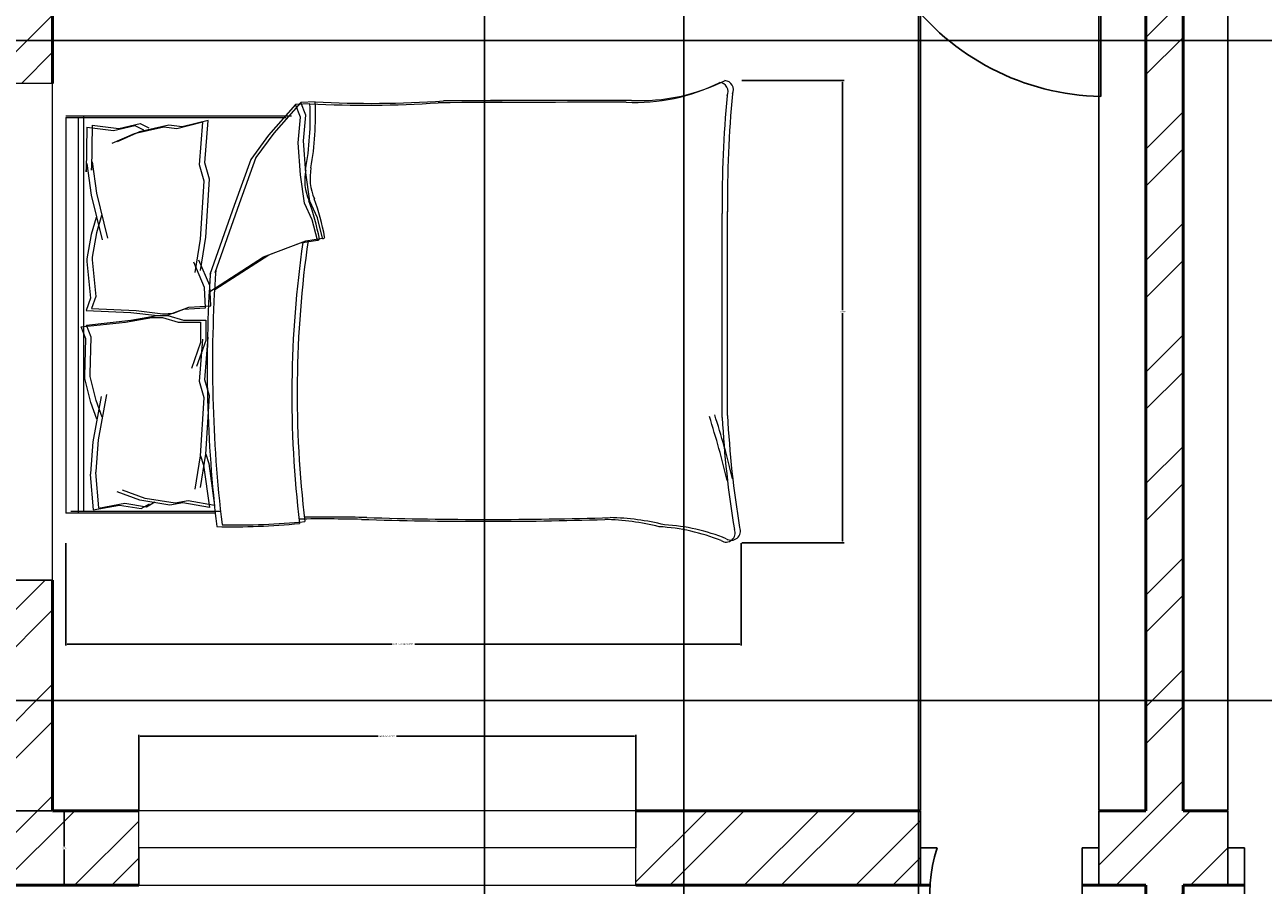
# Model space of a CAD drawing. Units: inches. Extents: x 1980 to 2738, y 1471 to 2568.
# Tile 3 of 22: x 2111 to 2260, y 1686 to 1790. Entities that reach past the tile are written whole.
import ezdxf

# ---------------------------------------------------------------- set-up
doc = ezdxf.new("R2010")
doc.units = ezdxf.units.IN
for name, color, linetype, lineweight in [('A-ANNO-DIMS', 2, 'Continuous', 18), ('A-DOOR', 31, 'Continuous', 25), ('A-FURN', 8, 'Continuous', 18), ('A-GLAZ', 141, 'Continuous', 18), ('A-WALL', 7, 'Continuous', 50)]:
    doc.layers.add(name, color=color, linetype=linetype, lineweight=lineweight)
doc.layers.add('A-WALL-PATT', color=9, linetype='Continuous', lineweight=13, true_color=0xd19cc7)
doc.styles.get("Standard").update_dxf_attribs({"font": 'arial.ttf'})
doc.dimstyles.get("Standard").update_dxf_attribs({"dimtxt": 0.18, "dimasz": 0.18, "dimexe": 0.18, "dimexo": 0.0625, "dimgap": 0.09, "dimtad": 0, "dimtih": 1, "dimtoh": 1, "dimdec": 4, "dimzin": 0, "dimdsep": 46, "dimtxsty": 'Standard', "dimcen": 0.09, "dimadec": 0, "dimazin": 0, "dimtfac": 1, "dimtdec": 4, "dimtofl": 0, "dimtmove": 0, "dimatfit": 3, "dimfxl": 1, "dimtolj": 1, "dimtzin": 0, "dimarcsym": 0})

# ---------------------------------------------------------------- blocks, each defined once
blk = doc.blocks.new('BED-DOUBLE')
for p, q in [((27.75, 52.87), (24.5, 49.16)), ((27.75, 52.87), (24.5, 49.16)), ((28.38, 53.1), (25.13, 49.39)), ((28.38, 53.1), (25.13, 49.39)), ((29.49, 52.95), (27.75, 52.87, 3.87)), ((29.49, 52.95), (27.75, 52.87, 3.87)), ((28.36, 51.33), (27.75, 52.87)), ((28.36, 51.33), (27.75, 52.87)), ((30.13, 53.18), (28.38, 53.1, 3.87)), ((30.13, 53.18), (28.38, 53.1, 3.87)), ((29, 51.56), (28.38, 53.1)), ((29, 51.56), (28.38, 53.1)), ((0, 51.49), (0.64, 51.49)), ((0, 51.27), (26.61, 51.27)), ((0, 51.27), (26.61, 51.27)), ((0, 51.27), (0, 3.48)), ((0.64, 51.49), (27.25, 51.49)), ((0.64, 51.49), (27.25, 51.49)), ((1.53, 3.48), (1.53, 51.27)), ((1.53, 3.48), (1.53, 51.27)), ((2.17, 3.7), (2.17, 51.49)), ((2.17, 3.7), (2.17, 51.49)), ((17.21, 50.93), (14.07, 50.15)), ((17.21, 50.93), (14.07, 50.15)), ((16.81, 45.8), (17.21, 50.93)), ((16.81, 45.79), (17.21, 50.93)), ((28.06, 48.23), (28.36, 51.33)), ((28.06, 48.23), (28.36, 51.33)), ((28.69, 48.46), (29, 51.56)), ((28.69, 48.46), (29, 51.56)), ((2.56, 50.11), (2.46, 44.71)), ((2.56, 50.11), (2.46, 44.71)), ((2.56, 50.11), (5.77, 49.73)), ((2.56, 50.11), (5.77, 49.73)), ((3.2, 50.34), (3.1, 44.94)), ((3.2, 50.34), (3.1, 44.94)), ((3.2, 50.34), (6.41, 49.96)), ((3.2, 50.34), (6.41, 49.96)), ((5.77, 49.73), (8.34, 50.33)), ((5.77, 49.73), (8.34, 50.33)), ((8.9, 49.54), (6.22, 48.36)), ((8.9, 49.54), (6.22, 48.36)), ((6.41, 49.96), (8.98, 50.56)), ((6.41, 49.96), (8.98, 50.56)), ((11.83, 50.11), (8.26, 49.31)), ((11.83, 50.11), (8.26, 49.31)), ((8.34, 50.33), (9.38, 49.81)), ((8.34, 50.33), (9.38, 49.81)), ((12.47, 50.34), (8.9, 49.54)), ((12.47, 50.34), (8.9, 49.54)), ((8.98, 50.56), (10.02, 50.04)), ((8.98, 50.56), (10.02, 50.04)), ((13.43, 49.92), (11.83, 50.11)), ((13.43, 49.92), (11.83, 50.11)), ((14.07, 50.15), (12.47, 50.34)), ((14.07, 50.15), (12.47, 50.34)), ((16.57, 50.7), (13.43, 49.92)), ((16.57, 50.7), (13.43, 49.92)), ((16.17, 45.57), (16.57, 50.7)), ((16.17, 45.57), (16.57, 50.7)), ((25.13, 49.39), (22.97, 46.45)), ((25.13, 49.39), (22.97, 46.45)), ((8.26, 49.31), (5.58, 48.13)), ((8.26, 49.31), (5.58, 48.13)), ((24.5, 49.16), (22.33, 46.22)), ((24.5, 49.16), (22.33, 46.22)), ((28.36, 44.36), (28.06, 48.23)), ((28.36, 44.36), (28.06, 48.23)), ((29, 44.59), (28.69, 48.46)), ((29, 44.59), (28.69, 48.46)), ((22.97, 46.45), (20.96, 40.87)), ((22.97, 46.45), (20.96, 40.87)), ((2.46, 44.71), (2.54, 45.71)), ((2.46, 44.71), (2.54, 45.71)), ((2.54, 45.71), (3.07, 41.91)), ((2.54, 45.71), (3.07, 41.91)), ((3.1, 44.94), (3.18, 45.94)), ((3.1, 44.94), (3.18, 45.94)), ((3.18, 45.94), (3.71, 42.14)), ((3.18, 45.94), (3.71, 42.14)), ((16.73, 43.61), (16.17, 45.57)), ((16.73, 43.61), (16.17, 45.57)), ((17.37, 43.83), (16.81, 45.8)), ((17.37, 43.83), (16.81, 45.79)), ((22.33, 46.22), (20.32, 40.64)), ((22.33, 46.22), (20.32, 40.64)), ((16.29, 36.6), (16.73, 43.61)), ((16.29, 36.6), (16.73, 43.61)), ((16.93, 36.82), (17.37, 43.83)), ((16.93, 36.82), (17.37, 43.83)), ((28.83, 40.95), (28.36, 44.36)), ((28.83, 40.95), (28.36, 44.36)), ((29.47, 41.18), (29, 44.59)), ((29.47, 41.18), (29, 44.59)), ((3.07, 41.91), (4.42, 36.5)), ((3.07, 41.91), (4.42, 36.5)), ((3.71, 42.14), (5.06, 36.72)), ((3.71, 42.14), (5.06, 36.72)), ((20.32, 40.64), (17.38, 32.31)), ((20.32, 40.64), (17.38, 32.31)), ((20.96, 40.87), (18.02, 32.53)), ((20.96, 40.87), (18.02, 32.53)), ((29.76, 38.94), (28.83, 40.95)), ((29.76, 38.94), (28.83, 40.95)), ((30.4, 39.17), (29.47, 41.18)), ((30.4, 39.17), (29.47, 41.18)), ((3.67, 39.2), (3.08, 37.14)), ((3.67, 39.2), (3.08, 37.14)), ((4.31, 39.43), (3.72, 37.36)), ((4.31, 39.43), (3.72, 37.36)), ((30.38, 36.46), (29.76, 38.94)), ((30.38, 36.46), (29.76, 38.94)), ((31.02, 36.69), (30.4, 39.17)), ((31.02, 36.69), (30.4, 39.17)), ((79.24, 15.06), (79.24, 39.68)), ((79.24, 15.06), (79.24, 39.68)), ((79.88, 15.29), (79.88, 39.91)), ((79.88, 15.29), (79.88, 39.91)), ((3.08, 37.14), (2.54, 34.2)), ((3.08, 37.14), (2.54, 34.2)), ((3.72, 37.36), (3.18, 34.43)), ((3.72, 37.36), (3.18, 34.43)), ((15.63, 32.56), (16.29, 36.6)), ((15.63, 32.56), (16.29, 36.6)), ((16.27, 32.79), (16.93, 36.82)), ((16.27, 32.79), (16.93, 36.82)), ((23.88, 34.45), (28.36, 36.15)), ((23.88, 34.45), (28.36, 36.15)), ((24.52, 34.68), (29, 36.38)), ((24.52, 34.68), (29, 36.38)), ((28.36, 36.15), (30.38, 36.46)), ((28.36, 36.15), (30.38, 36.46)), ((29, 36.38), (31.02, 36.69)), ((29, 36.38), (31.02, 36.69)), ((3.18, 34.43), (3.2, 34.11)), ((3.18, 34.43), (3.2, 34.11)), ((17.38, 30.26), (23.88, 34.45)), ((17.38, 30.26), (23.88, 34.45)), ((18.02, 30.49), (24.52, 34.68)), ((18.02, 30.49), (24.52, 34.68)), ((2.54, 34.2), (2.56, 33.88)), ((2.54, 34.2), (2.56, 33.88)), ((2.56, 33.88), (2.98, 29.46)), ((2.56, 33.88), (2.98, 29.46)), ((3.2, 34.11), (3.62, 29.68)), ((3.2, 34.11), (3.62, 29.68)), ((16.74, 30.75), (15.45, 33.82)), ((16.74, 30.75), (15.45, 33.82)), ((17.38, 30.98), (16.09, 34.05)), ((17.38, 30.98), (16.09, 34.05)), ((16.89, 28.3), (16.74, 30.75)), ((16.89, 28.3), (16.74, 30.75)), ((17.53, 28.53), (17.38, 30.98)), ((17.53, 28.53), (17.38, 30.98)), ((2.98, 29.46), (2.49, 27.98)), ((2.98, 29.46), (2.49, 27.98)), ((3.62, 29.68), (3.13, 28.21)), ((3.62, 29.68), (3.13, 28.21)), ((14.86, 28.36), (17.53, 28.53)), ((14.86, 28.36), (17.53, 28.53)), ((2.49, 27.98), (7.87, 27.73)), ((2.49, 27.98), (7.87, 27.73)), ((3.13, 28.21), (8.51, 27.96)), ((3.13, 28.21), (8.51, 27.96)), ((7.22, 26.56), (10.4, 27.14)), ((7.22, 26.56), (10.4, 27.14)), ((7.86, 26.79), (11.04, 27.37)), ((7.86, 26.79), (11.04, 27.37)), ((7.87, 27.73), (11.08, 27.36)), ((7.87, 27.73), (11.08, 27.35)), ((8.51, 27.96), (11.72, 27.58)), ((8.51, 27.96), (11.72, 27.58)), ((10.4, 27.14), (11.7, 27.14)), ((10.4, 27.14), (11.7, 27.14)), ((11.04, 27.37), (12.34, 27.37)), ((11.04, 27.37), (12.34, 27.37)), ((11.08, 27.36), (12.38, 27.44)), ((11.08, 27.35), (12.38, 27.44)), ((11.7, 27.14), (13.58, 26.56)), ((11.7, 27.14), (13.58, 26.56)), ((11.72, 27.58), (13.02, 27.66)), ((11.72, 27.58), (13.02, 27.66)), ((12.34, 27.37), (14.22, 26.79)), ((12.34, 27.37), (14.22, 26.79)), ((12.38, 27.44), (14.22, 28.13)), ((12.38, 27.44), (14.22, 28.13)), ((13.02, 27.66), (14.86, 28.36)), ((13.02, 27.66), (14.86, 28.36)), ((14.22, 28.13), (16.89, 28.3)), ((14.22, 28.13), (16.89, 28.3)), ((1.87, 25.98), (7.22, 26.56)), ((1.87, 25.98), (7.22, 26.56)), ((2.45, 24.54), (1.87, 25.98)), ((2.45, 24.54), (1.87, 25.98)), ((2.51, 26.21), (7.86, 26.79)), ((2.51, 26.21), (7.86, 26.79)), ((3.09, 24.77), (2.51, 26.21)), ((3.09, 24.77), (2.51, 26.21)), ((13.58, 26.56), (16.26, 26.56)), ((13.58, 26.56), (16.26, 26.56)), ((14.22, 26.79), (16.9, 26.79)), ((14.22, 26.79), (16.9, 26.79)), ((16.26, 26.56), (16.26, 24.1)), ((16.26, 26.56), (16.26, 24.1)), ((16.9, 26.79), (16.9, 24.33)), ((16.9, 26.79), (16.9, 24.33)), ((2.3, 20.09), (2.45, 24.54)), ((2.3, 20.09), (2.45, 24.54)), ((2.94, 20.32), (3.09, 24.77)), ((2.94, 20.32), (3.09, 24.77)), ((16.26, 24.1), (15.17, 20.96)), ((16.26, 24.1), (15.17, 20.96)), ((16.9, 24.33), (15.81, 21.19)), ((16.9, 24.33), (15.81, 21.19)), ((16.17, 19.38), (16.57, 24.52)), ((16.17, 19.38), (16.57, 24.52)), ((16.81, 19.61), (17.21, 24.74)), ((16.81, 19.61), (17.21, 24.74)), ((2.3, 19.77), (2.3, 20.09)), ((2.3, 19.77), (2.3, 20.09)), ((3.03, 16.88), (2.3, 19.77)), ((3.03, 16.88), (2.3, 19.77)), ((2.94, 20), (2.94, 20.32)), ((2.94, 20), (2.94, 20.32)), ((3.67, 17.11), (2.94, 20)), ((3.67, 17.11), (2.94, 20)), ((17.37, 17.65), (16.81, 19.61)), ((17.37, 17.65), (16.81, 19.61)), ((16.73, 17.42), (16.17, 19.38)), ((16.73, 17.42), (16.17, 19.38)), ((3.75, 14.86), (3.03, 16.88)), ((3.75, 14.85), (3.03, 16.88)), ((3.32, 12.11), (4.33, 17.6)), ((3.32, 12.11), (4.33, 17.6)), ((4.39, 15.08), (3.67, 17.11)), ((4.39, 15.08), (3.67, 17.11)), ((3.96, 12.34), (4.97, 17.83)), ((3.96, 12.34), (4.97, 17.83)), ((16.29, 10.41), (16.73, 17.42)), ((16.29, 10.41), (16.73, 17.42)), ((16.93, 10.64), (17.37, 17.65)), ((16.93, 10.64), (17.37, 17.65)), ((3.03, 8.29), (3.32, 12.11)), ((3.03, 8.28), (3.32, 12.11)), ((3.67, 8.51), (3.96, 12.34)), ((3.67, 8.51), (3.96, 12.34)), ((16.27, 6.61), (16.93, 10.64)), ((16.27, 6.61), (16.93, 10.64)), ((16.93, 10.64), (17.26, 9.51)), ((16.93, 10.64), (17.26, 9.51)), ((15.63, 6.38), (16.29, 10.41)), ((15.63, 6.38), (16.29, 10.41)), ((16.29, 10.41), (16.62, 9.28)), ((16.29, 10.41), (16.62, 9.28)), ((16.62, 9.28), (17.34, 4.18)), ((16.62, 9.28), (17.34, 4.18)), ((17.26, 9.51), (17.98, 4.41)), ((17.26, 9.51), (17.98, 4.41)), ((3.01, 8.18), (3.03, 8.29)), ((3.01, 8.18), (3.03, 8.28)), ((3.34, 3.9), (3.01, 8.18)), ((3.34, 3.9), (3.01, 8.18)), ((3.65, 8.41), (3.67, 8.51)), ((3.65, 8.41), (3.67, 8.51)), ((3.98, 4.13), (3.65, 8.41)), ((3.98, 4.13), (3.65, 8.41)), ((8.95, 5.05), (6.21, 6.06)), ((8.95, 5.05), (6.21, 6.06)), ((9.59, 5.28), (6.85, 6.29)), ((9.59, 5.28), (6.85, 6.29)), ((3.96, 4.12), (7.14, 4.7)), ((3.96, 4.12), (7.14, 4.7)), ((7.14, 4.7), (9.74, 4.27)), ((7.14, 4.7), (9.74, 4.27)), ((12.57, 4.47), (8.95, 5.05)), ((12.57, 4.47), (8.95, 5.05)), ((9.1, 4.04), (10.11, 4.62)), ((9.1, 4.04), (10.11, 4.62)), ((13.21, 4.7), (9.59, 5.28)), ((13.21, 4.7), (9.59, 5.28)), ((9.74, 4.27), (10.75, 4.85)), ((9.74, 4.27), (10.75, 4.85)), ((14.16, 4.76), (12.57, 4.47)), ((14.16, 4.76), (12.57, 4.47)), ((14.8, 4.99), (13.21, 4.7)), ((14.8, 4.99), (13.21, 4.7)), ((17.34, 4.18), (14.16, 4.76)), ((17.34, 4.18), (14.16, 4.76)), ((17.98, 4.41), (14.8, 4.99)), ((17.98, 4.41), (14.8, 4.99)), ((18.11, 3.48), (0, 3.48)), ((18.11, 3.48), (0, 3.48)), ((18.75, 3.7), (0.64, 3.7)), ((18.75, 3.7), (0.64, 3.7)), ((3.32, 3.89), (6.5, 4.47)), ((3.32, 3.89), (6.5, 4.47)), ((6.5, 4.47), (9.1, 4.04)), ((6.5, 4.47), (9.1, 4.04))]:
    blk.add_line(p, q)
for centre, radius, start, end in [((68.67, 76.16), 23.07, 267.4714, 296.4681), ((68.67, 76.16), 23.07, 267.4714, 296.4681), ((69.31, 76.39), 23.07, 267.4714, 296.4681), ((69.31, 76.39), 23.07, 267.4714, 296.4681), ((78.87, 54.41), 1.1, 332.6588, 86.02), ((78.87, 54.41), 1.1, 332.6588, 86.02), ((79.51, 54.64), 1.1, 332.6588, 86.02), ((79.51, 54.64), 1.1, 332.6588, 86.02), ((212.28, 41.15), 133.04, 174.4998, 180.6351), ((212.28, 41.15), 133.04, 174.4998, 180.6351), ((212.92, 41.38), 133.04, 174.4998, 180.6351), ((212.92, 41.38), 133.04, 174.4998, 180.6351), ((-6.66, 51.33), 36.18, 349.8763, 2.5657), ((-6.66, 51.33), 36.18, 349.8763, 2.5657), ((36.31, 182.27), 129.5, 266.9791, 273.8365), ((36.31, 182.27), 129.5, 266.9791, 273.8365), ((-6.02, 51.56), 36.18, 349.8763, 2.5657), ((-6.02, 51.56), 36.18, 349.8763, 2.5657), ((36.95, 182.49), 129.5, 266.9791, 273.8365), ((36.95, 182.49), 129.5, 266.9791, 273.8365), ((67.82, -4508.74), 4561.86, 90.00217, 90.28689), ((67.82, -4508.74), 4561.86, 90.00217, 90.28689), ((68.46, -4508.51), 4561.86, 90.00217, 90.28689), ((68.46, -4508.52), 4561.86, 90.00217, 90.28689), ((35.07, 43.74), 6.22, 168.6608, 203.7384), ((35.07, 43.74), 6.22, 168.6608, 203.7384), ((35.71, 43.97), 6.22, 168.6608, 203.7384), ((35.71, 43.97), 6.22, 168.6608, 203.7384), ((1.48, 31.15), 29.65, 10.6617, 19.8806), ((1.48, 31.15), 29.65, 10.6617, 19.8806), ((2.12, 31.38), 29.65, 10.6617, 19.8806), ((2.12, 31.38), 29.65, 10.6617, 19.8806), ((156.32, 17.76), 129.02, 171.7845, 186.9006), ((156.32, 17.76), 129.02, 171.7845, 186.9006), ((156.96, 17.98), 129.02, 171.7845, 186.9006), ((156.96, 17.98), 129.02, 171.7845, 186.9006), ((30.44, 36.64), 0.185, 250.2464, 1.1377), ((30.44, 36.64), 0.185, 250.2464, 1.1377), ((31.08, 36.86), 0.185, 250.2464, 1.1377), ((31.08, 36.86), 0.185, 250.2464, 1.1377), ((182.05, 21.36), 164.97, 176.0865, 186.7821), ((182.05, 21.36), 164.97, 176.0865, 186.7821), ((182.69, 21.59), 164.97, 176.0865, 186.7821), ((182.69, 21.59), 164.97, 176.0865, 186.7821), ((-23.71, -17.22), 106.46, 13.3832, 17.7053), ((-23.71, -17.22), 106.46, 13.3832, 17.7053), ((-23.07, -16.99), 106.46, 13.3832, 17.7053), ((-23.07, -16.99), 106.46, 13.3832, 17.7053), ((200.84, 21.43), 121.76, 182.9958, 189.4091), ((200.84, 21.43), 121.76, 182.9958, 189.4091), ((201.48, 21.66), 121.76, 182.9958, 189.4091), ((201.48, 21.66), 121.76, 182.9958, 189.4091), ((31.81, -167.08), 170.11, 88.4762, 91.0082), ((31.81, -167.08), 170.11, 88.4762, 91.0082), ((20.1, 85.16), 83.31, 268.7218, 275.604), ((20.1, 85.16), 83.31, 268.7218, 275.604), ((20.74, 85.39), 83.31, 268.7218, 275.604), ((20.74, 85.39), 83.31, 268.7218, 275.604), ((31.17, -167.31), 170.11, 88.4762, 91.0082), ((31.17, -167.31), 170.11, 88.4762, 91.0082), ((50.61, 484.82), 482.31, 268.2277, 271.7185), ((50.61, 484.82), 482.31, 268.2277, 271.7185), ((51.25, 485.05), 482.31, 268.2277, 271.7185), ((51.25, 485.05), 482.31, 268.2277, 271.7185), ((64.51, -26.9), 29.63, 76.0648, 88.9113), ((64.51, -26.9), 29.63, 76.0648, 88.9113), ((65.15, -26.67), 29.63, 76.0648, 88.9113), ((65.15, -26.67), 29.63, 76.0648, 88.9113), ((70.28, -21.66), 23.56, 67.9751, 86.652), ((70.28, -21.66), 23.56, 67.9751, 86.652), ((70.91, -21.43), 23.56, 67.9751, 86.652), ((70.91, -21.43), 23.56, 67.9751, 86.652), ((79.72, 1.09), 1.09, 236.1736, 23.4781), ((79.72, 1.09), 1.09, 236.1736, 23.4781), ((80.36, 1.32), 1.09, 236.1736, 23.4781), ((80.36, 1.32), 1.09, 236.1736, 23.4781)]:
    blk.add_arc(centre, radius, start, end)
blk = doc.blocks.new('WIN-60IN-WALL')
for p, q in [((0, 9), (0, 0)), ((60, 9), (0, 9)), ((60, 4.5), (60, 9)), ((60, 9), (60, 0)), ((0, 0), (0, 4.5)), ((0, 4.5), (60, 4.5)), ((0, 0), (60, 0))]:
    blk.add_line(p, q)
blk = doc.blocks.new('*D15')
at = {"layer": 'A-ANNO-DIMS', "color": 0, "lineweight": -2, "transparency": 16777216}
for p, q in [((2124.51, 1694.77), (2124.51, 1703.89)), ((2124.69, 1703.71), (2153.39, 1703.71)), ((2184.33, 1703.71), (2155.63, 1703.71)), ((2184.51, 1694.77), (2184.51, 1703.89))]:
    blk.add_line(p, q, dxfattribs=at)
at = {"layer": 'A-ANNO-DIMS', "color": 0, "transparency": 16777216}
for points in [[(2124.69, 1703.74), (2124.69, 1703.68), (2124.51, 1703.71)], [(2184.33, 1703.74), (2184.33, 1703.68), (2184.51, 1703.71)]]:
    blk.add_solid(points, dxfattribs=at)
at = {"layer": 'Defpoints', "color": 0, "transparency": 16777216}
for p in [(2124.51, 1703.71), (2124.51, 1694.71), (2184.51, 1694.71)]:
    blk.add_point(p, dxfattribs=at)
at = {"layer": 'A-ANNO-DIMS', "color": 0, "transparency": 16777216, "insert": (2154.51, 1703.71), "char_height": 0.18, "attachment_point": 5}
blk.add_mtext('\\A1;WINDOW 60 TYP.', dxfattribs=at)
blk = doc.blocks.new('*D16')
at = {"layer": 'A-ANNO-DIMS', "color": 0, "lineweight": -2, "transparency": 16777216}
for p, q in [((2124.45, 1694.71), (2115.33, 1694.71)), ((2115.51, 1694.53), (2115.51, 1690.39)), ((2115.51, 1685.89), (2115.51, 1690.02)), ((2124.45, 1685.71), (2115.33, 1685.71))]:
    blk.add_line(p, q, dxfattribs=at)
at = {"layer": 'A-ANNO-DIMS', "color": 0, "transparency": 16777216}
for points in [[(2115.48, 1694.53), (2115.54, 1694.53), (2115.51, 1694.71)], [(2115.48, 1685.89), (2115.54, 1685.89), (2115.51, 1685.71)]]:
    blk.add_solid(points, dxfattribs=at)
at = {"layer": 'Defpoints', "color": 0, "transparency": 16777216}
for p in [(2124.51, 1694.71), (2115.51, 1685.71), (2124.51, 1685.71)]:
    blk.add_point(p, dxfattribs=at)
at = {"layer": 'A-ANNO-DIMS', "color": 0, "transparency": 16777216, "insert": (2115.51, 1690.21), "char_height": 0.18, "attachment_point": 5}
blk.add_mtext('\\A1;9 TYP.', dxfattribs=at)
blk = doc.blocks.new('*D17')
at = {"layer": 'A-ANNO-DIMS', "color": 0, "lineweight": -2, "transparency": 16777216}
for p, q in [((2115.68, 1727), (2115.68, 1714.65)), ((2197.23, 1727), (2197.23, 1714.65)), ((2115.86, 1714.83), (2155.09, 1714.83)), ((2197.05, 1714.83), (2157.83, 1714.83))]:
    blk.add_line(p, q, dxfattribs=at)
at = {"layer": 'A-ANNO-DIMS', "color": 0, "transparency": 16777216}
for points in [[(2115.86, 1714.86), (2115.86, 1714.8), (2115.68, 1714.83)], [(2197.05, 1714.86), (2197.05, 1714.8), (2197.23, 1714.83)]]:
    blk.add_solid(points, dxfattribs=at)
at = {"layer": 'Defpoints', "color": 0, "transparency": 16777216}
for p in [(2115.68, 1727.06), (2197.23, 1727.06), (2197.23, 1714.83)]:
    blk.add_point(p, dxfattribs=at)
at = {"layer": 'A-ANNO-DIMS', "color": 0, "transparency": 16777216, "insert": (2156.46, 1714.83), "char_height": 0.18, "attachment_point": 5}
blk.add_mtext('\\A1;DOUBLE BED 82 TYP.', dxfattribs=at)
blk = doc.blocks.new('*D18')
at = {"layer": 'A-ANNO-DIMS', "color": 0, "lineweight": -2, "transparency": 16777216}
for p, q in [((2197.29, 1782.88), (2209.64, 1782.88)), ((2209.46, 1782.7), (2209.46, 1755.15)), ((2209.46, 1727.24), (2209.46, 1754.79)), ((2197.29, 1727.06), (2209.64, 1727.06))]:
    blk.add_line(p, q, dxfattribs=at)
at = {"layer": 'A-ANNO-DIMS', "color": 0, "transparency": 16777216}
for points in [[(2209.43, 1782.7), (2209.49, 1782.7), (2209.46, 1782.88)], [(2209.43, 1727.24), (2209.49, 1727.24), (2209.46, 1727.06)]]:
    blk.add_solid(points, dxfattribs=at)
at = {"layer": 'Defpoints', "color": 0, "transparency": 16777216}
for p in [(2197.23, 1782.88), (2209.46, 1782.88), (2197.23, 1727.06)]:
    blk.add_point(p, dxfattribs=at)
at = {"layer": 'A-ANNO-DIMS', "color": 0, "transparency": 16777216, "insert": (2209.46, 1754.97), "char_height": 0.18, "attachment_point": 5}
blk.add_mtext('\\A1;56 TYP.', dxfattribs=at)
blk = doc.blocks.new('*D40')
at = {"layer": 'A-ANNO-DIMS', "color": 0, "lineweight": -2, "transparency": 16777216}
for p, q in [((2218.65, 2053.14), (2218.65, 1533.71)), ((2298.65, 2053.14), (2298.65, 1533.71)), ((2218.83, 1533.89), (2258.43, 1533.89)), ((2298.47, 1533.89), (2258.87, 1533.89))]:
    blk.add_line(p, q, dxfattribs=at)
at = {"layer": 'A-ANNO-DIMS', "color": 0, "transparency": 16777216}
for points in [[(2218.83, 1533.92), (2218.83, 1533.86), (2218.65, 1533.89)], [(2298.47, 1533.92), (2298.47, 1533.86), (2298.65, 1533.89)]]:
    blk.add_solid(points, dxfattribs=at)
at = {"layer": 'Defpoints', "color": 0, "transparency": 16777216}
for p in [(2218.65, 2053.21), (2298.65, 2053.21), (2298.65, 1533.89)]:
    blk.add_point(p, dxfattribs=at)
at = {"layer": 'A-ANNO-DIMS', "color": 0, "transparency": 16777216, "insert": (2258.65, 1533.89), "char_height": 0.18, "attachment_point": 5}
blk.add_mtext('\\A1;80', dxfattribs=at)
blk = doc.blocks.new('*D44')
at = {"layer": 'A-ANNO-DIMS', "color": 0, "lineweight": -2, "transparency": 16777216}
for p, q in [((2218.88, 1694.77), (2218.88, 2507.54)), ((2219.06, 2507.36), (2229.18, 2507.36)), ((2240.22, 2507.36), (2230.11, 2507.36)), ((2240.4, 1694.77), (2240.4, 2507.54))]:
    blk.add_line(p, q, dxfattribs=at)
at = {"layer": 'A-ANNO-DIMS', "color": 0, "transparency": 16777216}
for points in [[(2219.06, 2507.39), (2219.06, 2507.33), (2218.88, 2507.36)], [(2240.22, 2507.39), (2240.22, 2507.33), (2240.4, 2507.36)]]:
    blk.add_solid(points, dxfattribs=at)
at = {"layer": 'Defpoints', "color": 0, "transparency": 16777216}
for p in [(2240.4, 2507.36), (2218.88, 1694.71), (2240.4, 1694.71)]:
    blk.add_point(p, dxfattribs=at)
at = {"layer": 'A-ANNO-DIMS', "color": 0, "transparency": 16777216, "insert": (2229.64, 2507.36), "char_height": 0.18, "attachment_point": 5}
blk.add_mtext('\\A1;21.525', dxfattribs=at)
blk = doc.blocks.new('*D45')
at = {"layer": 'A-ANNO-DIMS', "color": 0, "lineweight": -2, "transparency": 16777216}
for p, q in [((2255.99, 1694.77), (2255.99, 2507.54)), ((2256.17, 2507.36), (2267.22, 2507.36)), ((2279.21, 2507.36), (2268.15, 2507.36)), ((2279.39, 1694.77), (2279.39, 2507.54))]:
    blk.add_line(p, q, dxfattribs=at)
at = {"layer": 'A-ANNO-DIMS', "color": 0, "transparency": 16777216}
for points in [[(2256.17, 2507.39), (2256.17, 2507.33), (2255.99, 2507.36)], [(2279.21, 2507.39), (2279.21, 2507.33), (2279.39, 2507.36)]]:
    blk.add_solid(points, dxfattribs=at)
at = {"layer": 'Defpoints', "color": 0, "transparency": 16777216}
for p in [(2279.39, 2507.36), (2255.99, 1694.71), (2279.39, 1694.71)]:
    blk.add_point(p, dxfattribs=at)
at = {"layer": 'A-ANNO-DIMS', "color": 0, "transparency": 16777216, "insert": (2267.69, 2507.36), "char_height": 0.18, "attachment_point": 5}
blk.add_mtext('\\A1;23.407', dxfattribs=at)
blk = doc.blocks.new('*D47')
at = {"layer": 'A-ANNO-DIMS', "color": 0, "lineweight": -2, "transparency": 16777216}
for p, q in [((2166.25, 1814.64), (2166.25, 1533.71)), ((2190.3, 1814.64), (2190.3, 1533.71)), ((2166.43, 1533.89), (2177.81, 1533.89)), ((2190.12, 1533.89), (2178.74, 1533.89))]:
    blk.add_line(p, q, dxfattribs=at)
at = {"layer": 'A-ANNO-DIMS', "color": 0, "transparency": 16777216}
for points in [[(2166.43, 1533.92), (2166.43, 1533.86), (2166.25, 1533.89)], [(2190.12, 1533.92), (2190.12, 1533.86), (2190.3, 1533.89)]]:
    blk.add_solid(points, dxfattribs=at)
at = {"layer": 'Defpoints', "color": 0, "transparency": 16777216}
for p in [(2166.25, 1814.71), (2190.3, 1814.71), (2190.3, 1533.89)]:
    blk.add_point(p, dxfattribs=at)
at = {"layer": 'A-ANNO-DIMS', "color": 0, "transparency": 16777216, "insert": (2178.28, 1533.89), "char_height": 0.18, "attachment_point": 5}
blk.add_mtext('\\A1;24.044', dxfattribs=at)
blk = doc.blocks.new('*D49')
at = {"layer": 'A-ANNO-DIMS', "color": 0, "lineweight": -2, "transparency": 16777216}
for p, q in [((2105.02, 1722.55), (2036.25, 1722.55)), ((2036.43, 1722.37), (2036.43, 1708.81)), ((2036.43, 1694.89), (2036.43, 1708.45)), ((2114.02, 1694.71), (2036.25, 1694.71))]:
    blk.add_line(p, q, dxfattribs=at)
at = {"layer": 'A-ANNO-DIMS', "color": 0, "transparency": 16777216}
for points in [[(2036.4, 1722.37), (2036.46, 1722.37), (2036.43, 1722.55)], [(2036.4, 1694.89), (2036.46, 1694.89), (2036.43, 1694.71)]]:
    blk.add_solid(points, dxfattribs=at)
at = {"layer": 'Defpoints', "color": 0, "transparency": 16777216}
for p in [(2036.43, 1722.55), (2105.08, 1722.55), (2114.08, 1694.71)]:
    blk.add_point(p, dxfattribs=at)
at = {"layer": 'A-ANNO-DIMS', "color": 0, "transparency": 16777216, "insert": (2036.43, 1708.63), "char_height": 0.18, "attachment_point": 5}
blk.add_mtext('\\A1;27.845', dxfattribs=at)
blk = doc.blocks.new('*D52')
at = {"layer": 'A-ANNO-DIMS', "color": 0, "lineweight": -2, "transparency": 16777216}
for p, q in [((2341.71, 1787.71), (2036.25, 1787.71)), ((2036.43, 1787.53), (2036.43, 1748.05)), ((2036.43, 1708.21), (2036.43, 1747.69)), ((2341.71, 1708.03), (2036.25, 1708.03))]:
    blk.add_line(p, q, dxfattribs=at)
at = {"layer": 'A-ANNO-DIMS', "color": 0, "transparency": 16777216}
for points in [[(2036.4, 1787.53), (2036.46, 1787.53), (2036.43, 1787.71)], [(2036.4, 1708.21), (2036.46, 1708.21), (2036.43, 1708.03)]]:
    blk.add_solid(points, dxfattribs=at)
at = {"layer": 'Defpoints', "color": 0, "transparency": 16777216}
for p in [(2036.43, 1787.71), (2341.78, 1787.71), (2341.78, 1708.03)]:
    blk.add_point(p, dxfattribs=at)
at = {"layer": 'A-ANNO-DIMS', "color": 0, "transparency": 16777216, "insert": (2036.43, 1747.87), "char_height": 0.18, "attachment_point": 5}
blk.add_mtext('\\A1;79.68', dxfattribs=at)

msp = doc.modelspace()

# ---------------------------------------------------------------- hatches: boundary and pattern name
at = {"layer": 'A-WALL-PATT'}
h = msp.add_hatch(dxfattribs=at)
h.set_pattern_fill('ANSI32', color=256)
h.paths.add_polyline_path([(2257.5661, 2416.2064), (2257.5661, 2420.7064), (2250.5833, 2420.7064), (2250.5833, 2462.7064), (2246.0833, 2462.7064), (2246.0833, 2420.7064), (2237.0791, 2420.7064), (2237.0791, 2411.7064), (2246.0833, 2411.7064), (2246.0833, 2291.7064), (2242.6109, 2291.7064), (2242.6109, 2287.2064), (2246.0833, 2287.2064), (2250.5833, 2287.2064), (2250.5833, 2291.7064), (2250.5833, 2411.7064), (2257.5661, 2411.7064)])
h.paths.add_polyline_path([(2387.0396, 2416.2064), (2387.0396, 2420.7064), (2367.5833, 2420.7064), (2367.5833, 2462.7064), (2358.5833, 2462.7064), (2358.5833, 2420.7064), (2329.3087, 2420.7064), (2329.3087, 2411.7064), (2358.5833, 2411.7064), (2358.5833, 2321.7275), (2358.5833, 2309.7064), (2347.3089, 2309.7064), (2293.3089, 2309.7064), (2293.3089, 2259.0771), (2297.8089, 2259.0771), (2297.8089, 2305.2064), (2347.3089, 2305.2064), (2347.3089, 2284.7412), (2351.8089, 2284.7412), (2351.8089, 2305.2064), (2372.3188, 2305.2064), (2372.3761, 2284.3899), (2377.0295, 2284.3899), (2377.0295, 2299.3058), (2377.0295, 2305.2064), (2426.5295, 2305.2064), (2426.5295, 2257.5573), (2431.0295, 2257.5573), (2431.0295, 2309.7064), (2377.0295, 2309.7064), (2367.5833, 2309.7064), (2367.5833, 2321.7275), (2367.5833, 2411.7064), (2387.0396, 2411.7064)])
h.paths.add_polyline_path([(2448.5267, 2416.2064), (2448.5267, 2420.7064), (2423.0396, 2420.7064), (2423.0396, 2411.7064), (2448.5267, 2411.7064)])
h.paths.add_polyline_path([(2130.9128, 2416.2064), (2130.9128, 2420.7064), (2105.0833, 2420.7064), (2105.0833, 2386.6942), (2114.0833, 2386.6942), (2114.0833, 2411.7064), (2130.9128, 2411.7064)])
h.paths.add_polyline_path([(2212.9478, 2420.7064), (2190.9128, 2420.7064), (2190.9128, 2411.7064), (2212.9478, 2411.7064), (2212.9478, 2416.2064)])
h.paths.add_polyline_path([(2114.0833, 2326.6942), (2105.0833, 2326.6942), (2105.0833, 2291.7064), (2081.0833, 2291.7064), (2081.0833, 2287.2064), (2105.0833, 2287.2064), (2105.0833, 2276.1935), (2114.0833, 2276.1935), (2114.0833, 2287.2064), (2166.3825, 2287.2064), (2166.3825, 2289.4564), (2166.3825, 2291.7064), (2114.0833, 2291.7064)])
h.paths.add_polyline_path([(2114.0833, 2252.1935), (2105.0833, 2252.1935), (2105.0833, 2233.2064), (2081.0833, 2233.2064), (2081.0833, 2228.7064), (2105.0833, 2228.7064), (2105.0833, 2213.4478), (2114.0833, 2213.4478), (2114.0833, 2228.7064), (2195.0833, 2228.7064), (2199.5833, 2228.7064), (2208.4455, 2228.7064), (2208.4455, 2230.9564), (2208.4455, 2233.2064), (2199.5833, 2233.2064), (2199.5833, 2287.2064), (2206.8904, 2287.2064), (2206.8904, 2289.4564), (2206.8904, 2291.7064), (2189.446, 2291.7064), (2189.446, 2289.4564), (2189.446, 2287.2064), (2195.0833, 2287.2064), (2195.0833, 2233.2064), (2114.0833, 2233.2064)])
h.paths.add_polyline_path([(2114.0833, 2153.4478), (2109.5833, 2153.4478), (2105.0833, 2153.4478), (2105.0833, 2135.2374), (2114.0833, 2135.2374)], flags=17)
h.paths.add_polyline_path([(2135.9619, 2095.4081), (2140.1805, 2095.4081), (2140.1805, 2104.2064), (2114.0833, 2104.2064), (2114.0833, 2110.3997), (2109.5833, 2110.3997), (2105.0833, 2110.3997), (2105.0833, 2104.2064), (2081.0833, 2104.2064), (2081.0833, 2099.7064), (2105.0833, 2099.7064), (2127.5416, 2099.8532), (2127.5416, 2056.9393), (2136.2133, 2056.9393)], flags=17)
h.paths.add_polyline_path([(2255.4895, 2104.2064), (2250.5833, 2104.2064), (2250.5833, 2233.2064), (2246.0833, 2233.2064), (2242.4941, 2233.2064), (2242.4941, 2228.7064), (2246.0833, 2228.7064), (2246.0833, 2104.2064), (2163.6825, 2104.2064), (2163.6825, 2099.8072), (2163.6825, 2095.4081), (2191.4325, 2095.4081), (2191.4325, 2011.2064), (2186.0833, 2011.2064), (2136.5143, 2010.8824), (2136.3702, 2032.9403), (2131.9559, 2032.9115), (2127.5416, 2032.8826), (2127.5416, 2006.7064), (2105.0833, 2006.7064), (2081.0833, 2006.7064), (2081.0833, 2002.2064), (2105.0833, 2002.2064), (2105.0833, 1995.9329), (2114.0833, 1995.9329), (2114.0833, 2002.2064), (2246.0833, 2002.2064), (2246.0833, 1877.7064), (2242.1358, 1877.7064), (2242.1358, 1873.2064), (2250.5833, 1873.2064), (2250.5833, 2002.2064), (2255.3335, 2002.2064), (2255.3335, 2011.2064), (2195.9325, 2011.2064), (2195.9325, 2095.2064), (2255.4895, 2095.2064), (2255.4895, 2099.5471)])
h.paths.add_polyline_path([(2199.5833, 1873.2064), (2209.827, 1873.2064), (2209.827, 1875.4564), (2209.827, 1877.7064), (2114.0833, 1877.7064), (2114.0833, 1890.0968), (2105.0833, 1890.0968), (2105.0833, 1877.7064), (2081.0833, 1877.7064), (2081.0833, 1873.2064), (2105.0833, 1873.2064), (2105.0833, 1857.7279), (2114.0833, 1857.7279), (2114.0833, 1873.2064), (2195.0833, 1873.2064), (2195.0833, 1819.2064), (2190.298, 1819.2064), (2190.298, 1814.7064), (2209.8976, 1814.7064), (2209.8976, 1816.9564), (2209.8976, 1819.2064), (2199.5833, 1819.2064)])
h.paths.add_polyline_path([(2114.0833, 1814.7064), (2166.2538, 1814.7064), (2166.2538, 1816.9564), (2166.2538, 1819.2064), (2114.0833, 1819.2064), (2114.0833, 1833.7279), (2109.5833, 1833.7279), (2105.0833, 1833.7279), (2105.0833, 1819.2064), (2081.0833, 1819.2064), (2081.0833, 1814.7064), (2105.0833, 1814.7064), (2105.0833, 1782.5516), (2114.0833, 1782.5516)])
h.paths.add_polyline_path([(2114.0833, 1722.5516), (2109.5833, 1722.5516), (2105.0833, 1722.5516), (2105.0833, 1685.7064), (2124.5104, 1685.7064), (2124.5104, 1690.2064), (2124.5104, 1694.7064), (2114.0833, 1694.7064)])
h.paths.add_polyline_path([(2218.8787, 1694.7064), (2184.5104, 1694.7064), (2184.5104, 1685.7064), (2218.8787, 1685.7064), (2218.8787, 1690.2064)])
h.paths.add_polyline_path([(2250.5833, 1819.2064), (2242.6431, 1819.2064), (2242.6431, 1816.9564), (2242.6431, 1814.7064), (2246.0833, 1814.7064), (2246.0833, 1694.7064), (2240.4035, 1694.7064), (2240.4035, 1690.2064), (2240.4035, 1685.7064), (2246.0833, 1685.7064), (2246.0833, 1643.7064), (2250.5833, 1643.7064), (2250.5833, 1685.7064), (2255.9859, 1685.7064), (2255.9859, 1690.2064), (2255.9859, 1694.7064), (2250.5833, 1694.7064)])
h.paths.add_polyline_path([(2297.4764, 1694.7064), (2279.3934, 1694.7064), (2279.3934, 1690.2064), (2279.3934, 1685.7064), (2297.4764, 1685.7064), (2297.4764, 1690.2064)])
h.paths.add_polyline_path([(2377.1596, 1694.7064), (2367.5833, 1694.7064), (2367.5833, 1787.7064), (2431.0295, 1787.7064), (2431.0295, 1792.2064), (2431.0295, 1849.4149), (2428.7795, 1849.4149), (2426.5295, 1849.4149), (2426.5295, 1792.2064), (2421.5833, 1792.2064), (2367.5833, 1792.2064), (2297.8089, 1792.2064), (2297.8089, 1850.2946), (2295.5589, 1850.2946), (2293.3089, 1850.2946), (2293.3089, 1792.2064), (2293.3089, 1787.7064), (2297.8089, 1787.7064), (2358.5833, 1787.7064), (2358.5833, 1694.7064), (2333.4764, 1694.7064), (2333.4764, 1685.7064), (2358.5833, 1685.7064), (2358.5833, 1643.7064), (2367.5833, 1643.7064), (2367.5833, 1685.7064), (2377.1596, 1685.7064)])
h.paths.add_polyline_path([(2442.4912, 1694.7064), (2413.1596, 1694.7064), (2413.1596, 1685.7064), (2442.4912, 1685.7064)])
h.paths.add_polyline_path([(2480.0833, 1814.7064), (2483.4816, 1814.7064), (2483.4816, 1817.9384), (2483.4816, 1819.2064), (2475.5833, 1819.2064), (2475.5833, 1694.7064), (2470.7283, 1694.7064), (2470.7283, 1685.7064), (2475.5833, 1685.7064), (2475.5833, 1643.7064), (2480.0833, 1643.7064), (2480.0833, 1685.7064), (2486.3293, 1685.7064), (2486.3293, 1690.2064), (2486.3293, 1694.7064), (2480.0833, 1694.7064)])
h.paths.add_polyline_path([(2621.0833, 1721.7349), (2612.0833, 1721.7349), (2612.0833, 1694.7064), (2586.1453, 1694.7064), (2586.1453, 1685.7064), (2621.0833, 1685.7064)])
h.paths.add_polyline_path([(2526.1453, 1690.2064), (2526.1453, 1694.7064), (2511.584, 1694.7064), (2511.584, 1690.2064), (2511.584, 1685.7064), (2526.1453, 1685.7064)])
h.paths.add_polyline_path([(2645.0833, 1819.2064), (2621.0833, 1819.2064), (2621.0833, 1835.8527), (2616.5833, 1835.8527), (2612.0833, 1835.8527), (2612.0833, 1819.2064), (2560.2541, 1819.2064), (2560.2541, 1814.7064), (2612.0833, 1814.7064), (2612.0833, 1781.7349), (2621.0833, 1781.7349), (2621.0833, 1814.7064), (2645.0833, 1814.7064)])
h.paths.add_polyline_path([(2645.0833, 1877.7064), (2621.0833, 1877.7064), (2621.0833, 1886.4375), (2612.0833, 1886.4375), (2612.0833, 1877.7064), (2517.1032, 1877.7064), (2517.1032, 1875.4564), (2517.1032, 1873.2064), (2526.5833, 1873.2064), (2526.5833, 1819.2064), (2516.6454, 1819.2064), (2516.6454, 1816.9564), (2516.6454, 1814.7064), (2536.4445, 1814.7064), (2536.4445, 1816.9564), (2536.4445, 1819.2064), (2531.0833, 1819.2064), (2531.0833, 1873.2064), (2612.0833, 1873.2064), (2612.0833, 1859.8527), (2621.0833, 1859.8527), (2621.0833, 1873.2064), (2645.0833, 1873.2064)])
h.paths.add_polyline_path([(2645.0833, 2006.7064), (2621.0833, 2006.7064), (2588.5085, 2006.7064), (2588.5085, 2052.9125), (2579.9045, 2052.9125), (2579.9045, 2011.2064), (2519.9045, 2011.2064), (2519.9045, 2095.2064), (2553.1204, 2095.2064), (2553.1204, 2104.2064), (2480.0833, 2104.2064), (2480.0833, 2228.7064), (2484.3832, 2228.7064), (2484.3832, 2230.9564), (2484.3832, 2233.2064), (2475.5833, 2233.2064), (2475.5833, 2104.2064), (2463.1308, 2104.2064), (2463.1308, 2095.2064), (2501.2463, 2095.2064), (2510.9045, 2095.2064), (2515.4045, 2095.2064), (2515.4045, 2011.2064), (2510.9045, 2011.2064), (2501.2463, 2011.2064), (2462.5957, 2011.2064), (2462.5957, 2002.2064), (2475.5833, 2002.2064), (2475.5833, 1873.2064), (2483.6146, 1873.2064), (2483.6146, 1875.4564), (2483.6146, 1877.7064), (2480.0833, 1877.7064), (2480.0833, 2002.2064), (2612.0833, 2002.2064), (2612.0833, 1996.309), (2621.0833, 1996.309), (2621.0833, 2002.2064), (2645.0833, 2002.2064)])
h.paths.add_polyline_path([(2588.5085, 2099.7277), (2621.0833, 2099.7277), (2645.0833, 2099.7064), (2645.0833, 2104.2064), (2621.0833, 2104.2064), (2621.0833, 2109.0038), (2616.5833, 2109.0038), (2612.0833, 2109.0038), (2612.0833, 2104.2064), (2575.0621, 2104.2064), (2575.0621, 2099.7064), (2575.0621, 2095.2064), (2579.9045, 2095.2064), (2579.9045, 2076.9125), (2588.5085, 2076.9125)], flags=17)
h.paths.add_polyline_path([(2367.5833, 2002.2064), (2373.7228, 2002.2064), (2373.7228, 2006.7064), (2373.7228, 2011.2064), (2350.7889, 2011.2064), (2350.7889, 2006.7064), (2350.7889, 2002.2064), (2358.5833, 2002.2064), (2358.5833, 1877.7064), (2293.3089, 1877.7064), (2293.3089, 1870.4987), (2297.8089, 1870.4987), (2297.8089, 1873.2064), (2347.3089, 1873.2064), (2347.3089, 1847.2208), (2351.8089, 1847.2208), (2351.8089, 1873.2064), (2372.5295, 1873.2064), (2372.5295, 1847.8619), (2377.0295, 1847.8619), (2377.0295, 1873.2064), (2426.5295, 1873.2064), (2426.5295, 1868.7339), (2431.0295, 1868.7339), (2431.0295, 1877.7064), (2367.5833, 1877.7064)])
h.paths.add_polyline_path([(2531.0833, 2287.2064), (2534.2285, 2287.2064), (2534.2285, 2291.7064), (2516.7886, 2291.7064), (2516.7886, 2287.2064), (2526.5833, 2287.2064), (2526.5833, 2233.2064), (2517.9112, 2233.2064), (2517.9112, 2230.9564), (2517.9112, 2228.7064), (2526.5833, 2228.7064), (2531.0833, 2228.7064), (2612.0833, 2228.7064), (2612.0833, 2206.8504), (2621.0833, 2206.8504), (2621.0833, 2228.7064), (2645.0833, 2228.7064), (2645.0833, 2233.2064), (2621.0833, 2233.2064), (2621.0833, 2241.8536), (2616.5833, 2241.8536), (2612.0833, 2241.8536), (2612.0833, 2233.2064), (2531.0833, 2233.2064)])
h.paths.add_polyline_path([(2645.0833, 2291.7064), (2621.0833, 2291.7064), (2621.0833, 2323.0138), (2616.5833, 2323.0138), (2612.0833, 2323.0138), (2612.0833, 2291.7064), (2559.6852, 2291.7064), (2559.6852, 2289.4564), (2559.6852, 2287.2064), (2612.0833, 2287.2064), (2612.0833, 2265.8536), (2621.0833, 2265.8536), (2621.0833, 2287.2064), (2645.0833, 2287.2064)])
h.paths.add_polyline_path([(2621.0833, 2420.7064), (2582.8189, 2420.7064), (2582.8189, 2411.7064), (2612.0833, 2411.7064), (2612.0833, 2383.0138), (2621.0833, 2383.0138)])
h.paths.add_polyline_path([(2480.0833, 2411.7064), (2485.7342, 2411.7064), (2485.7342, 2416.2064), (2485.7342, 2420.7064), (2480.0833, 2420.7064), (2480.0833, 2462.7064), (2475.5833, 2462.7064), (2475.5833, 2420.7064), (2469.4083, 2420.7064), (2469.4083, 2411.7064), (2475.5833, 2411.7064), (2475.5833, 2291.7064), (2475.5833, 2287.2064), (2482.9195, 2287.2064), (2482.9195, 2289.4564), (2482.9195, 2291.7064), (2480.0833, 2291.7064)])
h.paths.add_polyline_path([(2367.5833, 2228.7064), (2431.0295, 2228.7064), (2431.0295, 2233.2064), (2431.0295, 2237.4203), (2428.7795, 2237.4203), (2426.5295, 2237.4203), (2426.5295, 2233.2064), (2377.0295, 2233.2064), (2377.0295, 2260.3837), (2372.4423, 2260.3837), (2372.517, 2233.2635), (2351.8089, 2233.2064), (2351.8089, 2260.7412), (2347.3089, 2260.7412), (2347.3089, 2233.2064), (2297.8089, 2233.2064), (2297.8089, 2236.9324), (2293.3089, 2236.9324), (2293.3089, 2228.7064), (2358.5833, 2228.7064), (2358.5833, 2104.2064), (2353.3665, 2104.2064), (2353.3665, 2095.2064), (2373.8869, 2095.2064), (2373.8869, 2099.7064), (2373.8869, 2104.2064), (2367.5833, 2104.2064)])
h.paths.add_polyline_path([(2321.2323, 2104.2064), (2303.4895, 2104.2064), (2303.4895, 2095.2064), (2321.2323, 2095.2064), (2321.2323, 2099.7064)], flags=0)
h.paths.add_polyline_path([(2415.1308, 2099.7064), (2415.1308, 2104.2064), (2404.81, 2104.2064), (2404.81, 2095.2064), (2415.1308, 2095.2064)], flags=17)
h.paths.add_polyline_path([(2318.6336, 2011.2064), (2303.3335, 2011.2064), (2303.3335, 2002.2064), (2318.6336, 2002.2064)], flags=0)
h.paths.add_polyline_path([(2414.5957, 2011.2064), (2406.2461, 2011.2064), (2406.2461, 2006.7064), (2406.2461, 2002.2064), (2414.5957, 2002.2064)], flags=17)

# ---------------------------------------------------------------- linework, layer by layer
at = {"layer": 'A-DOOR'}
for p, q in [((2240.6431, 1816.9564), (2240.6431, 1780.9564)), ((2218.8787, 1694.7064), (2218.8787, 1685.7064)), ((2240.4035, 1685.7064), (2240.4035, 1694.7064)), ((2240.4035, 1694.7064), (2240.4035, 1690.2064)), ((2255.9859, 1694.7064), (2255.9859, 1685.7064)), ((2218.8787, 1685.7064), (2218.8787, 1690.2064)), ((2218.8787, 1690.2064), (2220.8787, 1690.2064)), ((2240.4035, 1690.2064), (2238.4035, 1690.2064)), ((2238.4035, 1690.2064), (2238.4035, 1666.2064)), ((2255.9859, 1685.7064), (2255.9859, 1690.2064)), ((2255.9859, 1690.2064), (2257.9859, 1690.2064)), ((2257.9859, 1690.2064), (2257.9859, 1666.2064))]:
    msp.add_line(p, q, dxfattribs=at)
for centre, radius, start, end in [((2241.2573, 1810.9233), 29.9732, 163.957397, 268.825814), ((2238.4035, 1684.6047), 18.3983, 162.273895, 270), ((2257.9859, 1686.0533), 19.8469, 270, 12.078851)]:
    msp.add_arc(centre, radius, start, end, dxfattribs=at)
at = {"layer": 'A-GLAZ'}
msp.add_line((2124.5104, 1694.7064), (2124.5104, 1694.7064), dxfattribs=at)
at = {"layer": 'A-WALL'}
for p, q in [((2250.5833, 1819.2064), (2250.5833, 1694.7064)), ((2114.0833, 1814.7064), (2114.0833, 1782.5516)), ((2246.0833, 1814.7064), (2246.0833, 1694.7064)), ((2114.0833, 1722.5516), (2114.0833, 1694.7064)), ((2124.5104, 1694.7064), (2114.0833, 1694.7064)), ((2218.8787, 1694.7064), (2184.5104, 1694.7064)), ((2246.0833, 1694.7064), (2240.4035, 1694.7064)), ((2255.9859, 1694.7064), (2250.5833, 1694.7064)), ((2124.5104, 1685.7064), (2105.0833, 1685.7064)), ((2220.0382, 1685.7064), (2184.5104, 1685.7064)), ((2246.0833, 1685.7064), (2238.4035, 1685.7064)), ((2246.0833, 1685.7064), (2246.0833, 1643.7064)), ((2250.5833, 1685.7064), (2250.5833, 1643.7064)), ((2257.9859, 1685.7064), (2250.5833, 1685.7064))]:
    msp.add_line(p, q, dxfattribs=at)

# ---------------------------------------------------------------- block references
at = {"layer": 'A-FURN'}
msp.add_blockref('BED-DOUBLE', (2115.6836, 1727.1456), dxfattribs=at)
at = {"layer": 'A-GLAZ'}
for p, rotation in [((2105.0828, 1782.5514), 270), ((2184.5101, 1694.7068), 180)]:
    msp.add_blockref('WIN-60IN-WALL', p, dxfattribs=dict(at, rotation=rotation))

# ---------------------------------------------------------------- dimensions: what is measured, and where the dimension line sits
at = {"layer": 'A-ANNO-DIMS'}
for base, p1, p2, override, picture, middle in [((2240.4035, 2507.3564), (2218.8787, 1694.7064), (2240.4035, 1694.7064), {"dimdec": 3, "dimlfac": 1, "dimrnd": 0, "dimzin": 0, "dimdsep": 46, "dimlunit": 2}, '*D44', (2229.6411, 2507.3564)), ((2279.39337, 2507.35642), (2255.98588, 1694.70642), (2279.39337, 1694.70642), {"dimdec": 3, "dimlfac": 1, "dimrnd": 0, "dimzin": 0, "dimdsep": 46, "dimlunit": 2}, '*D45', (2267.68962, 2507.35642)), ((2298.6516, 1533.8857), (2218.6516, 2053.2064), (2298.6516, 2053.2064), {"dimdec": 0, "dimlfac": 1, "dimrnd": 0, "dimzin": 0, "dimdsep": 46, "dimlunit": 2}, '*D40', (2258.6516, 1533.8857)), ((2190.298, 1533.8857), (2166.2538, 1814.7064), (2190.298, 1814.7064), {"dimdec": 3, "dimlfac": 1, "dimrnd": 0, "dimzin": 0, "dimdsep": 46, "dimlunit": 2}, '*D47', (2178.2759, 1533.8857))]:
    dim = msp.add_linear_dim(base=base, p1=p1, p2=p2, dimstyle='Standard', override=override, dxfattribs=at)
    dim.commit()
    dim.dimension.update_dxf_attribs({"geometry": picture, "text_midpoint": middle})
for base, p1, p2, override, picture, middle in [((2036.4333, 1787.7064), (2341.776, 1708.0291), (2341.776, 1787.7064), {"dimdec": 2, "dimlfac": 1, "dimrnd": 0, "dimzin": 0, "dimdsep": 46, "dimlunit": 2}, '*D52', (2036.4333, 1747.8678)), ((2036.4333, 1722.5516), (2114.0833, 1694.7064), (2105.0833, 1722.5516), {"dimdec": 3, "dimlfac": 1, "dimrnd": 0, "dimzin": 0, "dimdsep": 46, "dimlunit": 2}, '*D49', (2036.4333, 1708.629))]:
    dim = msp.add_linear_dim(base=base, p1=p1, p2=p2, angle=90, dimstyle='Standard', override=override, dxfattribs=at)
    dim.commit()
    dim.dimension.update_dxf_attribs({"geometry": picture, "text_midpoint": middle})
for base, p1, p2, angle, text, picture, middle in [((2209.4642, 1782.8839), (2197.2319, 1727.0594), (2197.2319, 1782.8839), 90, '<> TYP.', '*D18', (2209.4642, 1754.9717)), ((2124.5104, 1703.7064), (2184.5104, 1694.7064), (2124.5104, 1694.7064), 180, 'WINDOW <> TYP.', '*D15', (2154.5104, 1703.7064)), ((2115.5104, 1685.7064), (2124.5104, 1694.7064), (2124.5104, 1685.7064), 270, '<> TYP.', '*D16', (2115.5104, 1690.2064))]:
    dim = msp.add_linear_dim(base=base, p1=p1, p2=p2, angle=angle, text=text, dimstyle='Standard', override={"dimdec": 0, "dimlfac": 1, "dimrnd": 0, "dimzin": 0, "dimdsep": 46, "dimlunit": 2}, dxfattribs=at)
    dim.commit()
    dim.dimension.update_dxf_attribs({"geometry": picture, "text_midpoint": middle})
dim = msp.add_linear_dim(base=(2197.2319, 1714.8271), p1=(2115.6833, 1727.0594), p2=(2197.2319, 1727.0594), text='DOUBLE BED <> TYP.', dimstyle='Standard', override={"dimdec": 0, "dimlfac": 1, "dimrnd": 0, "dimzin": 0, "dimdsep": 46, "dimlunit": 2}, dxfattribs=at)
dim.commit()
dim.dimension.update_dxf_attribs({"geometry": '*D17', "text_midpoint": (2156.4576, 1714.8271)})

doc.saveas('drawing.dxf')
